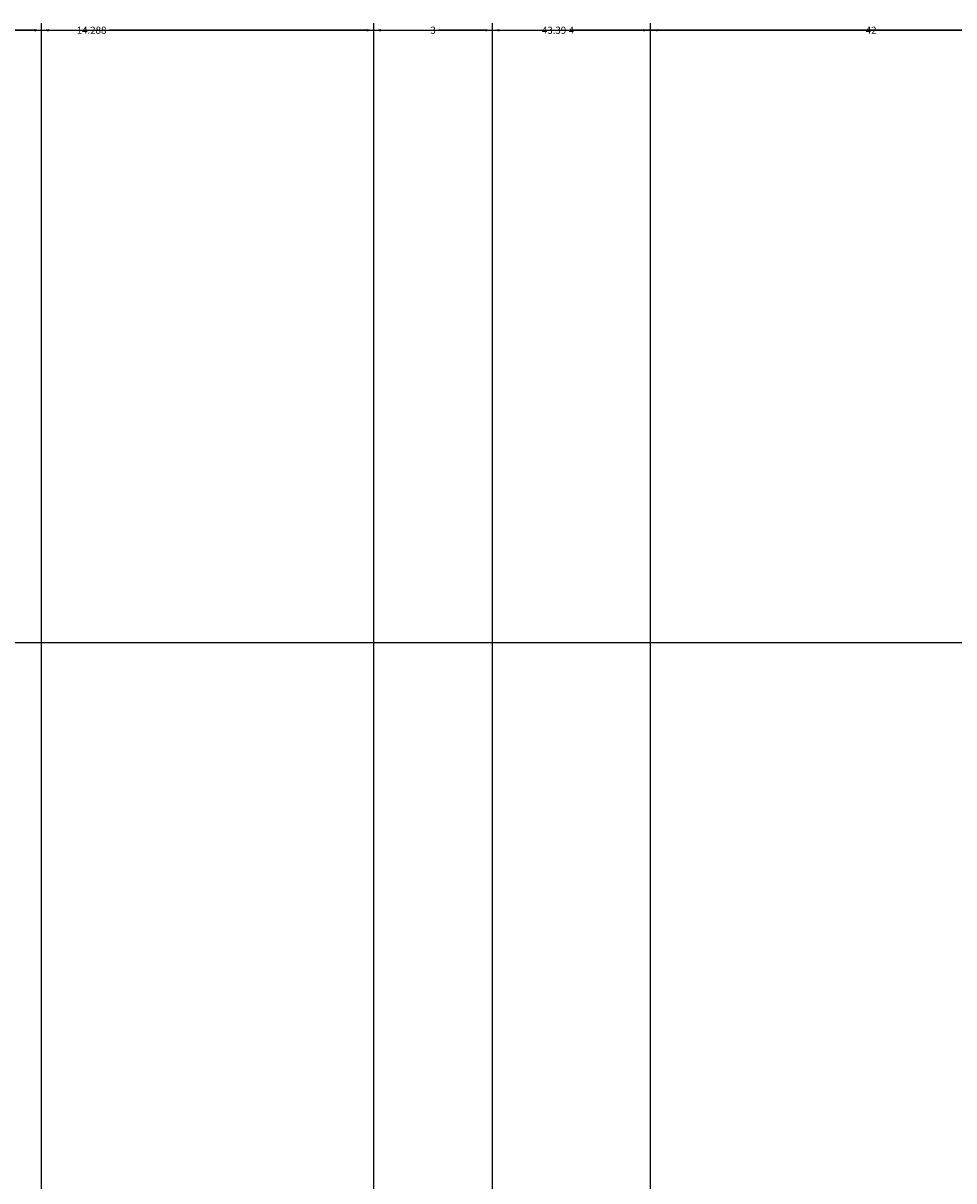
# Model space of a CAD drawing. Units: inches. Extents: x -6 to 289, y -8 to 323.
# Tile 88 of 107: x 126 to 150, y 294 to 323. Entities that reach past the tile are written whole.
import ezdxf

# ---------------------------------------------------------------- set-up
doc = ezdxf.new("R2010")
doc.units = ezdxf.units.IN
doc.header["$MEASUREMENT"] = 0
doc.layers.add('A-ANNO-DIMS', color=2, linetype='Continuous', lineweight=18)
doc.styles.get("Standard").update_dxf_attribs({"font": 'arial.ttf'})
doc.dimstyles.get("Standard").update_dxf_attribs({"dimtxt": 0.18, "dimasz": 0.18, "dimexe": 0.18, "dimexo": 0.0625, "dimgap": 0.09, "dimtad": 0, "dimtih": 1, "dimtoh": 1, "dimdec": 4, "dimzin": 0, "dimdsep": 46, "dimtxsty": 'Standard', "dimcen": 0.09, "dimadec": 0, "dimazin": 0, "dimtfac": 1, "dimtdec": 4, "dimtofl": 0, "dimtmove": 0, "dimatfit": 3, "dimfxl": 1, "dimtolj": 1, "dimtzin": 0, "dimarcsym": 0})

# ---------------------------------------------------------------- blocks, each defined once
blk = doc.blocks.new('*D10')
at = {"layer": 'A-ANNO-DIMS', "color": 0, "lineweight": -2, "transparency": 16777216}
for p, q in [((115.164, 307.351), (115.164, 322.969)), ((126.883, 226.717), (126.883, 322.969)), ((115.344, 322.789), (120.639, 322.789)), ((126.703, 322.789), (121.408, 322.789))]:
    blk.add_line(p, q, dxfattribs=at)
at = {"layer": 'A-ANNO-DIMS', "color": 0, "transparency": 16777216}
for points in [[(115.344, 322.819), (115.344, 322.759), (115.164, 322.789)], [(126.703, 322.819), (126.703, 322.759), (126.883, 322.789)]]:
    blk.add_solid(points, dxfattribs=at)
at = {"layer": 'Defpoints', "color": 0, "transparency": 16777216}
for p in [(126.883, 322.789), (115.164, 307.289), (126.883, 226.654)]:
    blk.add_point(p, dxfattribs=at)
at = {"layer": 'A-ANNO-DIMS', "color": 0, "transparency": 16777216, "insert": (121.024, 322.789), "char_height": 0.18, "attachment_point": 5}
blk.add_mtext('\\A1;11.72', dxfattribs=at)
blk = doc.blocks.new('*D11')
at = {"layer": 'A-ANNO-DIMS', "color": 0, "lineweight": -2, "transparency": 16777216}
for p, q in [((126.883, 226.717), (126.883, 322.969)), ((168.883, 226.717), (168.883, 322.969)), ((127.063, 322.789), (147.662, 322.789)), ((168.703, 322.789), (148.105, 322.789))]:
    blk.add_line(p, q, dxfattribs=at)
at = {"layer": 'A-ANNO-DIMS', "color": 0, "transparency": 16777216}
for points in [[(127.063, 322.819), (127.063, 322.759), (126.883, 322.789)], [(168.703, 322.819), (168.703, 322.759), (168.883, 322.789)]]:
    blk.add_solid(points, dxfattribs=at)
at = {"layer": 'Defpoints', "color": 0, "transparency": 16777216}
for p in [(168.883, 322.789), (126.883, 226.654), (168.883, 226.654)]:
    blk.add_point(p, dxfattribs=at)
at = {"layer": 'A-ANNO-DIMS', "color": 0, "transparency": 16777216, "insert": (147.883, 322.789), "char_height": 0.18, "attachment_point": 5}
blk.add_mtext('\\A1;42', dxfattribs=at)
blk = doc.blocks.new('*D27')
at = {"layer": 'A-ANNO-DIMS', "color": 0, "lineweight": -2, "transparency": 16777216}
for p, q in [((19.226, 307.289), (288.653, 307.289)), ((288.473, 307.109), (288.473, 277.471)), ((288.473, 247.469), (288.473, 277.107)), ((247.226, 247.289), (288.653, 247.289))]:
    blk.add_line(p, q, dxfattribs=at)
at = {"layer": 'A-ANNO-DIMS', "color": 0, "transparency": 16777216}
for points in [[(288.443, 307.109), (288.503, 307.109), (288.473, 307.289)], [(288.443, 247.469), (288.503, 247.469), (288.473, 247.289)]]:
    blk.add_solid(points, dxfattribs=at)
at = {"layer": 'Defpoints', "color": 0, "transparency": 16777216}
for p in [(19.164, 307.289), (288.473, 307.289), (247.164, 247.289)]:
    blk.add_point(p, dxfattribs=at)
at = {"layer": 'A-ANNO-DIMS', "color": 0, "transparency": 16777216, "insert": (288.473, 277.289), "char_height": 0.18, "attachment_point": 5}
blk.add_mtext('\\A1;60', dxfattribs=at)
blk = doc.blocks.new('*D73')
at = {"layer": 'A-ANNO-DIMS', "color": 0, "lineweight": -2, "transparency": 16777216}
for p, q in [((121.008, 51.148), (121.008, 322.969)), ((135.296, 51.148), (135.296, 322.969)), ((121.188, 322.789), (127.697, 322.789)), ((135.116, 322.789), (128.607, 322.789))]:
    blk.add_line(p, q, dxfattribs=at)
at = {"layer": 'A-ANNO-DIMS', "color": 0, "transparency": 16777216}
for points in [[(121.188, 322.819), (121.188, 322.759), (121.008, 322.789)], [(135.116, 322.819), (135.116, 322.759), (135.296, 322.789)]]:
    blk.add_solid(points, dxfattribs=at)
at = {"layer": 'Defpoints', "color": 0, "transparency": 16777216}
for p in [(135.296, 322.789), (121.008, 51.085), (135.296, 51.085)]:
    blk.add_point(p, dxfattribs=at)
at = {"layer": 'A-ANNO-DIMS', "color": 0, "transparency": 16777216, "insert": (128.152, 322.789), "char_height": 0.18, "attachment_point": 5}
blk.add_mtext('\\A1;14.288', dxfattribs=at)
blk = doc.blocks.new('*D74')
at = {"layer": 'A-ANNO-DIMS', "color": 0, "lineweight": -2, "transparency": 16777216}
for p, q in [((135.296, 51.148), (135.296, 322.969)), ((138.296, 51.148), (138.296, 322.969)), ((135.476, 322.789), (136.647, 322.789)), ((138.116, 322.789), (136.945, 322.789))]:
    blk.add_line(p, q, dxfattribs=at)
at = {"layer": 'A-ANNO-DIMS', "color": 0, "transparency": 16777216}
for points in [[(135.476, 322.819), (135.476, 322.759), (135.296, 322.789)], [(138.116, 322.819), (138.116, 322.759), (138.296, 322.789)]]:
    blk.add_solid(points, dxfattribs=at)
at = {"layer": 'Defpoints', "color": 0, "transparency": 16777216}
for p in [(138.296, 322.789), (135.296, 51.085), (138.296, 51.085)]:
    blk.add_point(p, dxfattribs=at)
at = {"layer": 'A-ANNO-DIMS', "color": 0, "transparency": 16777216, "insert": (136.796, 322.789), "char_height": 0.18, "attachment_point": 5}
blk.add_mtext('\\A1;3', dxfattribs=at)
blk = doc.blocks.new('*D75')
at = {"layer": 'A-ANNO-DIMS', "color": 0, "lineweight": -2, "transparency": 16777216}
for p, q in [((138.296, 51.148), (138.296, 322.969)), ((142.296, 51.148), (142.296, 322.969)), ((138.476, 322.789), (140.144, 322.789)), ((142.116, 322.789), (140.448, 322.789))]:
    blk.add_line(p, q, dxfattribs=at)
at = {"layer": 'A-ANNO-DIMS', "color": 0, "transparency": 16777216}
for points in [[(138.476, 322.819), (138.476, 322.759), (138.296, 322.789)], [(142.116, 322.819), (142.116, 322.759), (142.296, 322.789)]]:
    blk.add_solid(points, dxfattribs=at)
at = {"layer": 'Defpoints', "color": 0, "transparency": 16777216}
for p in [(142.296, 322.789), (138.296, 51.085), (142.296, 51.085)]:
    blk.add_point(p, dxfattribs=at)
at = {"layer": 'A-ANNO-DIMS', "color": 0, "transparency": 16777216, "insert": (140.296, 322.789), "char_height": 0.18, "attachment_point": 5}
blk.add_mtext('\\A1;4', dxfattribs=at)
blk = doc.blocks.new('*D76')
at = {"layer": 'A-ANNO-DIMS', "color": 0, "lineweight": -2, "transparency": 16777216}
for p, q in [((142.296, 51.148), (142.296, 322.969)), ((164.296, 51.148), (164.296, 322.969)), ((142.476, 322.789), (153.076, 322.789)), ((164.116, 322.789), (153.516, 322.789))]:
    blk.add_line(p, q, dxfattribs=at)
at = {"layer": 'A-ANNO-DIMS', "color": 0, "transparency": 16777216}
for points in [[(142.476, 322.819), (142.476, 322.759), (142.296, 322.789)], [(164.116, 322.819), (164.116, 322.759), (164.296, 322.789)]]:
    blk.add_solid(points, dxfattribs=at)
at = {"layer": 'Defpoints', "color": 0, "transparency": 16777216}
for p in [(164.296, 322.789), (142.296, 51.085), (164.296, 51.085)]:
    blk.add_point(p, dxfattribs=at)
at = {"layer": 'A-ANNO-DIMS', "color": 0, "transparency": 16777216, "insert": (153.296, 322.789), "char_height": 0.18, "attachment_point": 5}
blk.add_mtext('\\A1;22', dxfattribs=at)
blk = doc.blocks.new('*D94')
at = {"layer": 'A-ANNO-DIMS', "color": 0, "lineweight": -2, "transparency": 16777216}
for p, q in [((118.164, 159.411), (118.164, 322.969)), ((161.552, 159.411), (161.552, 322.969)), ((118.344, 322.789), (139.46, 322.789)), ((161.372, 322.789), (140.256, 322.789))]:
    blk.add_line(p, q, dxfattribs=at)
at = {"layer": 'A-ANNO-DIMS', "color": 0, "transparency": 16777216}
for points in [[(118.344, 322.819), (118.344, 322.759), (118.164, 322.789)], [(161.372, 322.819), (161.372, 322.759), (161.552, 322.789)]]:
    blk.add_solid(points, dxfattribs=at)
at = {"layer": 'Defpoints', "color": 0, "transparency": 16777216}
for p in [(161.552, 322.789), (118.164, 159.348), (161.552, 159.348)]:
    blk.add_point(p, dxfattribs=at)
at = {"layer": 'A-ANNO-DIMS', "color": 0, "transparency": 16777216, "insert": (139.858, 322.789), "char_height": 0.18, "attachment_point": 5}
blk.add_mtext('\\A1;43.39', dxfattribs=at)
blk = doc.blocks.new('*D107')
at = {"layer": 'A-ANNO-DIMS', "color": 0, "lineweight": -2, "transparency": 16777216}
for p, q in [((118.164, 293.728), (118.164, 322.969)), ((186.984, 291.541), (186.984, 322.969)), ((118.344, 322.789), (152.18, 322.789)), ((186.804, 322.789), (152.967, 322.789))]:
    blk.add_line(p, q, dxfattribs=at)
at = {"layer": 'A-ANNO-DIMS', "color": 0, "transparency": 16777216}
for points in [[(118.344, 322.819), (118.344, 322.759), (118.164, 322.789)], [(186.804, 322.819), (186.804, 322.759), (186.984, 322.789)]]:
    blk.add_solid(points, dxfattribs=at)
at = {"layer": 'Defpoints', "color": 0, "transparency": 16777216}
for p in [(186.984, 322.789), (118.164, 293.666), (186.984, 291.478)]:
    blk.add_point(p, dxfattribs=at)
at = {"layer": 'A-ANNO-DIMS', "color": 0, "transparency": 16777216, "insert": (152.574, 322.789), "char_height": 0.18, "attachment_point": 5}
blk.add_mtext('\\A1;68.82', dxfattribs=at)
blk = doc.blocks.new('*D118')
at = {"layer": 'A-ANNO-DIMS', "color": 0, "lineweight": -2, "transparency": 16777216}
for p, q in [((118.226, 307.289), (288.653, 307.289)), ((288.473, 307.109), (288.473, 300.659)), ((288.473, 293.846), (288.473, 300.295)), ((257.703, 293.666), (288.653, 293.666))]:
    blk.add_line(p, q, dxfattribs=at)
at = {"layer": 'A-ANNO-DIMS', "color": 0, "transparency": 16777216}
for points in [[(288.443, 307.109), (288.503, 307.109), (288.473, 307.289)], [(288.443, 293.846), (288.503, 293.846), (288.473, 293.666)]]:
    blk.add_solid(points, dxfattribs=at)
at = {"layer": 'Defpoints', "color": 0, "transparency": 16777216}
for p in [(118.164, 307.289), (288.473, 307.289), (257.641, 293.666)]:
    blk.add_point(p, dxfattribs=at)
at = {"layer": 'A-ANNO-DIMS', "color": 0, "transparency": 16777216, "insert": (288.473, 300.477), "char_height": 0.18, "attachment_point": 5}
blk.add_mtext('\\A1;13.623', dxfattribs=at)

msp = doc.modelspace()

# ---------------------------------------------------------------- dimensions: what is measured, and where the dimension line sits
at = {"layer": 'A-ANNO-DIMS'}
for base, p1, p2, override, picture, middle in [((126.8835, 322.7888), (115.1638, 307.2888), (126.8835, 226.654), {"dimdec": 2, "dimlfac": 1, "dimrnd": 0, "dimzin": 0, "dimdsep": 46, "dimlunit": 2}, '*D10', (121.0236, 322.7888)), ((161.5522, 322.7888), (118.1638, 159.3484), (161.5522, 159.3484), {"dimdec": 2, "dimlfac": 1, "dimrnd": 0, "dimzin": 0, "dimdsep": 46, "dimlunit": 2}, '*D94', (139.858, 322.7888)), ((186.9837, 322.7888), (118.1638, 293.6657), (186.9837, 291.4781), {"dimdec": 2, "dimlfac": 1, "dimrnd": 0, "dimzin": 0, "dimdsep": 46, "dimlunit": 2}, '*D107', (152.5737, 322.7888)), ((135.296, 322.7888), (121.008, 51.0851), (135.296, 51.0851), {"dimdec": 3, "dimlfac": 1, "dimrnd": 0, "dimzin": 0, "dimdsep": 46, "dimlunit": 2}, '*D73', (128.152, 322.7888)), ((168.8835, 322.7888), (126.8835, 226.654), (168.8835, 226.654), {"dimdec": 0, "dimlfac": 1, "dimrnd": 0, "dimzin": 0, "dimdsep": 46, "dimlunit": 2}, '*D11', (147.8835, 322.7888)), ((138.296, 322.7888), (135.296, 51.0851), (138.296, 51.0851), {"dimdec": 0, "dimlfac": 1, "dimrnd": 0, "dimzin": 0, "dimdsep": 46, "dimlunit": 2}, '*D74', (136.796, 322.7888)), ((142.296, 322.7888), (138.296, 51.0851), (142.296, 51.0851), {"dimdec": 0, "dimlfac": 1, "dimrnd": 0, "dimzin": 0, "dimdsep": 46, "dimlunit": 2}, '*D75', (140.296, 322.7888)), ((164.296, 322.7888), (142.296, 51.0851), (164.296, 51.0851), {"dimdec": 0, "dimlfac": 1, "dimrnd": 0, "dimzin": 0, "dimdsep": 46, "dimlunit": 2}, '*D76', (153.296, 322.7888))]:
    dim = msp.add_linear_dim(base=base, p1=p1, p2=p2, dimstyle='Standard', override=override, dxfattribs=at)
    dim.commit()
    dim.dimension.update_dxf_attribs({"geometry": picture, "text_midpoint": middle})
for p1, p2, override, picture, middle in [((247.1638, 247.2888), (19.1638, 307.2888), {"dimdec": 0, "dimlfac": 1, "dimrnd": 0, "dimzin": 0, "dimdsep": 46, "dimlunit": 2}, '*D27', (288.4733, 277.2888)), ((257.6407, 293.6657), (118.1638, 307.2888), {"dimdec": 3, "dimlfac": 1, "dimrnd": 0, "dimzin": 0, "dimdsep": 46, "dimlunit": 2}, '*D118', (288.4733, 300.4773))]:
    dim = msp.add_linear_dim(base=(288.4733, 307.2888), p1=p1, p2=p2, angle=90, dimstyle='Standard', override=override, dxfattribs=at)
    dim.commit()
    dim.dimension.update_dxf_attribs({"geometry": picture, "text_midpoint": middle})

doc.saveas('drawing.dxf')
